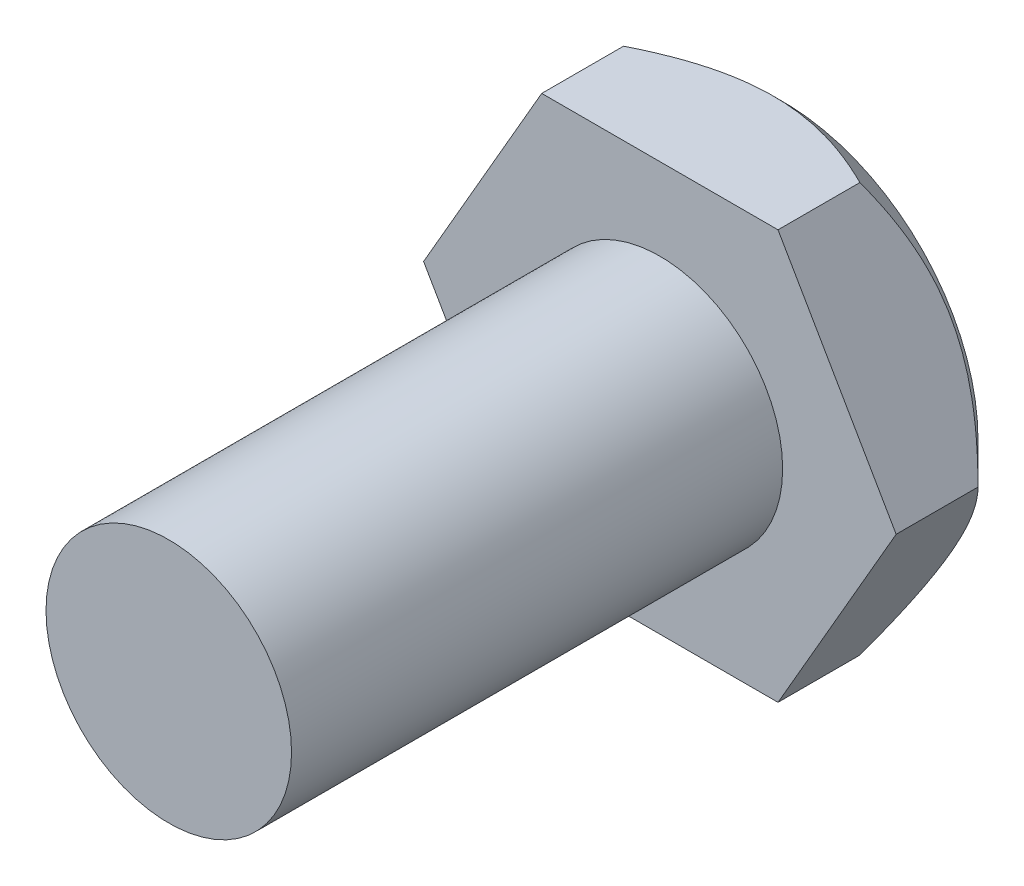
from build123d import *

# Parameters (mm, degrees)
HEX_HEAD_DEPTH    = 3
SHANK_PROFILE_6_R = 3
SHANK_6X12_DEPTH  = 12


with BuildPart() as part:
    # Hex Head Profile 10AF → Hex Head (new body)
    with BuildSketch(Plane.XY):
        Polygon((-2.886751346, 5), (-5.773502692, 0), (-2.886751346, -5), (2.886751346, -5), (5.773502692, 0), (2.886751346, 5), align=None)
    extrude(amount=HEX_HEAD_DEPTH)

    # Shank Profile Ø6 → Shank Ø6x12 (add)
    with BuildSketch(Plane.XY.offset(3)):
        Circle(SHANK_PROFILE_6_R)
    extrude(amount=SHANK_6X12_DEPTH)

    # Head Chamfer Profile → Head Chamfer 45x1 (revolve, cut)
    with BuildSketch(Plane(origin=(0, 0, 0), x_dir=(1, 0, 0), z_dir=(0, 1, 0)), mode=Mode.PRIVATE) as head_chamfer_45x1_sk:
        Polygon((-4.773502692, 0), (-5.773502692, 0), (-5.773502692, -1), align=None)
    revolve(head_chamfer_45x1_sk.sketch.rotate(Axis((0, 0, -2.775923962), (0, 0, 1)), 180), axis=Axis((0, 0, -2.775923962), (0, 0, 1)), mode=Mode.SUBTRACT)


solid = part.part
